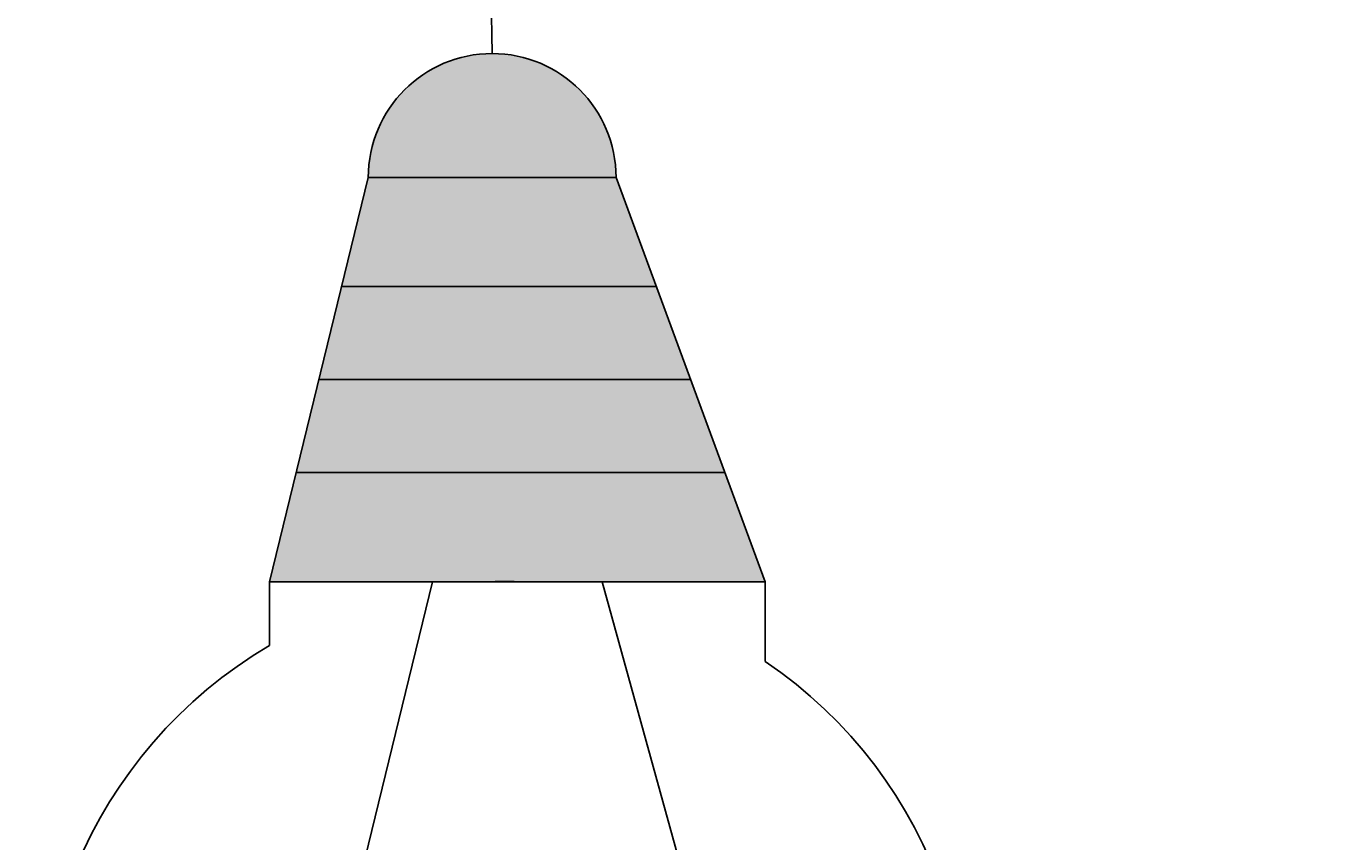
# Model space of a CAD drawing. Units: millimetres. Extents: x -8 to 285, y 5 to 221.
# Tile 24 of 30: x 130 to 172, y 159 to 185. Entities that reach past the tile are written whole.
import ezdxf

# ---------------------------------------------------------------- set-up
doc = ezdxf.new("R2010")
doc.units = ezdxf.units.MM
for name, color, linetype, lineweight in [('A-ANNO-DIMS', 2, 'Continuous', 18), ('E-EQPM-PATT', 252, 'Continuous', 13), ('E-LITE-FIXT', 7, 'Continuous', 25)]:
    doc.layers.add(name, color=color, linetype=linetype, lineweight=lineweight)
doc.layers.add('E-POWR-AC-LINE', color=30, linetype='Continuous', lineweight=25, true_color=0xf26722)
doc.styles.get("Standard").update_dxf_attribs({"font": 'arial.ttf'})
doc.dimstyles.get("Standard").update_dxf_attribs({"dimtxt": 0.18, "dimasz": 0.18, "dimexe": 0.18, "dimexo": 0.0625, "dimgap": 0.09, "dimtad": 0, "dimtih": 1, "dimtoh": 1, "dimdec": 4, "dimzin": 0, "dimdsep": 46, "dimtxsty": 'Standard', "dimcen": 0.09, "dimadec": 0, "dimazin": 0, "dimtfac": 1, "dimtdec": 4, "dimtofl": 0, "dimtmove": 0, "dimatfit": 3, "dimfxl": 1, "dimtolj": 1, "dimtzin": 0, "dimarcsym": 0})

# ---------------------------------------------------------------- blocks, each defined once
blk = doc.blocks.new('LAMP-INCANDESCENT')
for p, q in [((7.407, 29.994), (10.595, 43.039)), ((23.407, 29.994), (18.595, 43.039)), ((9.734, 39.517), (19.894, 39.517)), ((9.001, 36.517), (21.001, 36.517)), ((8.268, 33.517), (22.107, 33.517)), ((7.407, 29.994), (7.407, 27.935)), ((12.666, 29.994), (8.834, 14.293)), ((22.321, 14.903), (18.146, 29.994)), ((23.407, 29.994), (23.407, 27.423)), ((8.834, 14.293), (13.574, 17.029)), ((13.574, 17.029), (17.067, 15.012)), ((17.067, 15.012), (18.333, 17.205)), ((18.333, 17.205), (22.321, 14.903))]:
    blk.add_line(p, q)
for points in [[(10.595, 43.039), (18.595, 43.039)], [(23.407, 29.994), (7.407, 29.994)]]:
    blk.add_lwpolyline(points)
for centre, radius, start, end in [((14.595, 43.039), 4, 0, 180), ((15.001, 15), 15, 88.4488, 91.5512), ((15.001, 15), 15, 120.4152, 55.9163)]:
    blk.add_arc(centre, radius, start, end)
blk = doc.blocks.new('*D9')
at = {"layer": 'A-ANNO-DIMS', "color": 0, "lineweight": -2, "transparency": 16777216}
for p, q in [((6.672, 133.79), (6.672, 220.737)), ((6.852, 220.557), (138.33, 220.557)), ((270.739, 220.557), (139.262, 220.557)), ((270.919, 206.519), (270.919, 220.737))]:
    blk.add_line(p, q, dxfattribs=at)
at = {"layer": 'A-ANNO-DIMS', "color": 0, "transparency": 16777216}
for points in [[(6.852, 220.587), (6.852, 220.527), (6.672, 220.557)], [(270.739, 220.587), (270.739, 220.527), (270.919, 220.557)]]:
    blk.add_solid(points, dxfattribs=at)
at = {"layer": 'Defpoints', "color": 0, "transparency": 16777216}
for p in [(270.919, 220.557), (270.919, 206.457), (6.672, 133.727)]:
    blk.add_point(p, dxfattribs=at)
at = {"layer": 'A-ANNO-DIMS', "color": 0, "transparency": 16777216, "insert": (138.796, 220.557), "char_height": 0.18, "attachment_point": 5}
blk.add_mtext('\\A1;264.25', dxfattribs=at)
blk = doc.blocks.new('*D10')
at = {"layer": 'A-ANNO-DIMS', "color": 0, "lineweight": -2, "transparency": 16777216}
for p, q in [((145.103, 206.457), (-7.608, 206.457)), ((-7.428, 206.277), (-7.428, 113.161)), ((-7.428, 19.682), (-7.428, 112.797)), ((30.453, 19.502), (-7.608, 19.502))]:
    blk.add_line(p, q, dxfattribs=at)
at = {"layer": 'A-ANNO-DIMS', "color": 0, "transparency": 16777216}
for points in [[(-7.458, 206.277), (-7.398, 206.277), (-7.428, 206.457)], [(-7.458, 19.682), (-7.398, 19.682), (-7.428, 19.502)]]:
    blk.add_solid(points, dxfattribs=at)
at = {"layer": 'Defpoints', "color": 0, "transparency": 16777216}
for p in [(-7.428, 206.457), (145.165, 206.457), (30.516, 19.502)]:
    blk.add_point(p, dxfattribs=at)
at = {"layer": 'A-ANNO-DIMS', "color": 0, "transparency": 16777216, "insert": (-7.428, 112.979), "char_height": 0.18, "attachment_point": 5}
blk.add_mtext('\\A1;186.95', dxfattribs=at)

msp = doc.modelspace()

# ---------------------------------------------------------------- hatches: boundary and pattern name
at = {"layer": 'E-EQPM-PATT'}
h = msp.add_hatch(color=256, dxfattribs=at)
h.set_gradient(color1=(0, 0, 255), color2=(34, 52, 110), tint=1)
h.paths.add_polyline_path([(141.2836, 180.1071), (149.2836, 180.1071, 1)])
h.paths.add_polyline_path([(149.2836, 180.1071), (141.2836, 180.1071), (140.4228, 176.5846), (150.583, 176.5846)])
h.paths.add_polyline_path([(150.583, 176.5846), (140.4228, 176.5846), (139.6897, 173.5846), (151.6897, 173.5846)])
h.paths.add_polyline_path([(151.6897, 173.5846), (139.6897, 173.5846), (138.9565, 170.5846), (152.7963, 170.5846)])
h.paths.add_polyline_path([(152.7963, 170.5846), (138.9565, 170.5846), (138.0957, 167.062), (145.2836, 167.062, -0.0135377), (146.0957, 167.062), (154.0957, 167.062)])
h.paths.add_polyline_path([(193.1131, 180.1071), (185.1131, 180.1071), (184.2522, 176.5846), (194.4125, 176.5846)])
h.paths.add_polyline_path([(185.1131, 180.1071), (193.1131, 180.1071, 1)])
h.paths.add_polyline_path([(194.4125, 176.5846), (184.2522, 176.5846), (183.5191, 173.5846), (195.5191, 173.5846)])
h.paths.add_polyline_path([(195.5191, 173.5846), (183.5191, 173.5846), (182.786, 170.5846), (196.6258, 170.5846)])
h.paths.add_polyline_path([(196.6258, 170.5846), (182.786, 170.5846), (181.9252, 167.062), (189.1131, 167.062, -0.0135377), (189.9252, 167.062), (197.9252, 167.062)])
h.paths.add_polyline_path([(227.0413, 180.1071), (235.0413, 180.1071, 1)])
h.paths.add_polyline_path([(235.0413, 180.1071), (227.0413, 180.1071), (226.1804, 176.5846), (236.3407, 176.5846)])
h.paths.add_polyline_path([(236.3407, 176.5846), (226.1804, 176.5846), (225.4473, 173.5846), (237.4473, 173.5846)])
h.paths.add_polyline_path([(237.4473, 173.5846), (225.4473, 173.5846), (224.7142, 170.5846), (238.554, 170.5846)])
h.paths.add_polyline_path([(238.554, 170.5846), (224.7142, 170.5846), (223.8534, 167.062), (231.0413, 167.062, -0.0135377), (231.8534, 167.062), (239.8534, 167.062)])
h = msp.add_hatch(color=256, dxfattribs=at)
h.set_gradient(color2=(0, 0, 0), tint=1)
h.paths.add_polyline_path([(149.2836, 180.1071, 1), (141.2836, 180.1071)])
h.paths.add_polyline_path([(193.1131, 180.1071, 1), (185.1131, 180.1071)])
h.paths.add_polyline_path([(227.0413, 180.1071), (235.0413, 180.1071, 1)])

# ---------------------------------------------------------------- linework, layer by layer
at = {"layer": 'E-POWR-AC-LINE'}
msp.add_line((145.2836, 184.1071), (145.1651, 191.4908), dxfattribs=at)

# ---------------------------------------------------------------- block references
at = {"layer": 'E-LITE-FIXT'}
msp.add_blockref('LAMP-INCANDESCENT', (130.689, 137.068), dxfattribs=at)

# ---------------------------------------------------------------- dimensions: what is measured, and where the dimension line sits
at = {"layer": 'A-ANNO-DIMS'}
dim = msp.add_linear_dim(base=(270.9192, 220.5568), p1=(6.6725, 133.7273), p2=(270.9192, 206.4568), dimstyle='Standard', override={"dimdec": 2, "dimlfac": 1, "dimrnd": 0, "dimzin": 0, "dimdsep": 46, "dimlunit": 2}, dxfattribs=at)
dim.commit()
dim.dimension.update_dxf_attribs({"geometry": '*D9', "text_midpoint": (138.7958, 220.5568)})
dim = msp.add_linear_dim(base=(-7.4275, 206.4568), p1=(30.516, 19.502), p2=(145.1651, 206.4568), angle=90, dimstyle='Standard', override={"dimdec": 2, "dimlfac": 1, "dimrnd": 0, "dimzin": 0, "dimdsep": 46, "dimlunit": 2}, dxfattribs=at)
dim.commit()
dim.dimension.update_dxf_attribs({"geometry": '*D10', "text_midpoint": (-7.4275, 112.9794)})

doc.saveas('drawing.dxf')
